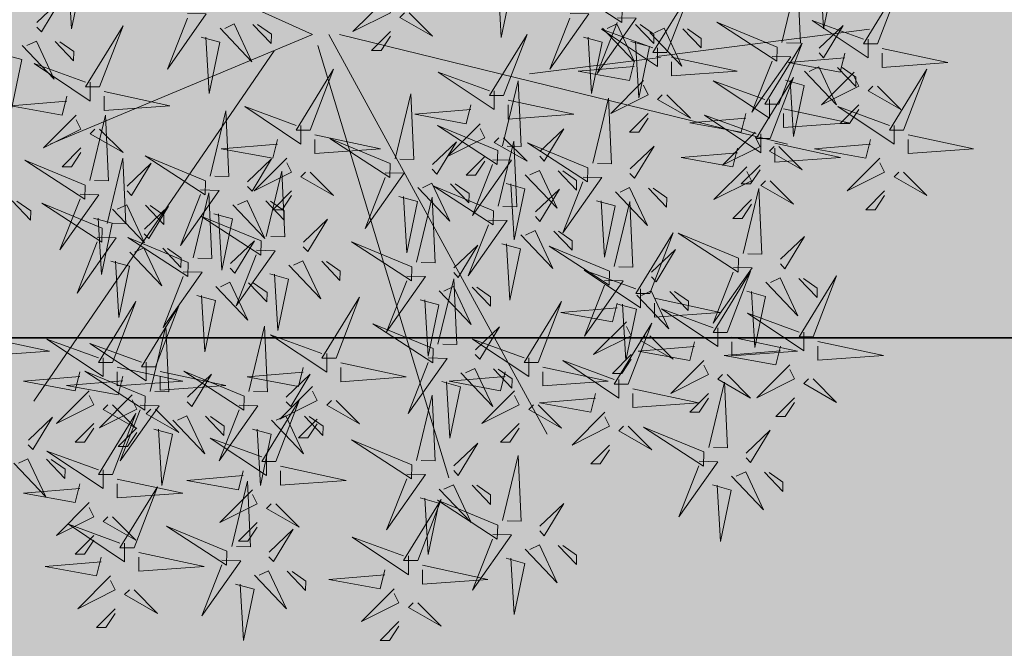
# Model space of a CAD drawing. Units: inches. Extents: x 1704 to 6393, y -157 to 1172.
# Tile 55 of 122: x 1906 to 1931, y 887 to 903. Entities that reach past the tile are written whole.
import ezdxf

# ---------------------------------------------------------------- set-up
doc = ezdxf.new("R2010")
doc.units = ezdxf.units.IN
doc.header["$MEASUREMENT"] = 0
for name, color, linetype, lineweight in [('A-ANNO-DIMS', 7, 'Continuous', 13), ('L-shrub', 74, 'Continuous', 18), ('WALLS', 7, 'Continuous', 35)]:
    doc.layers.add(name, color=color, linetype=linetype, lineweight=lineweight)
doc.layers.add('L-HRDS-PATT', color=9, linetype='Continuous', lineweight=13, true_color=0xc5c1ba)
doc.styles.get("Standard").update_dxf_attribs({"font": 'arial.ttf'})
doc.dimstyles.get("Standard").update_dxf_attribs({"dimtxt": 6, "dimasz": 2, "dimexe": 0.18, "dimexo": 0.0625, "dimgap": 0.09, "dimtad": 0, "dimtih": 1, "dimtoh": 1, "dimdec": 1, "dimzin": 0, "dimdsep": 46, "dimlunit": 3, "dimtxsty": 'Standard', "dimblk": 'ARCHTICK', "dimcen": 0.09, "dimadec": 0, "dimazin": 0, "dimtfac": 1, "dimtdec": 1, "dimtofl": 0, "dimtmove": 0, "dimatfit": 3, "dimfxl": 1, "dimtolj": 1, "dimtzin": 0, "dimarcsym": 0})

# ---------------------------------------------------------------- blocks, each defined once
blk = doc.blocks.new('shrub3')
for p, q in [((-5.99, -2.5), (58.67, 140.12)), ((-14.08, 16.34), (-186.51, 134.74)), ((-5.99, -2.5), (-59.88, 126.66)), ((-11.38, -5.19), (-224.23, -69.78)), ((-5.99, -10.57), (-202.68, -118.21)), ((-5.99, -15.96), (-59.88, -236.62)), ((-17.27, -174.02), (-25.36, -109.43)), ((-16.77, -172.03), (-3.3, -276.98))]:
    blk.add_line(p, q)
for points in [[(-154.93, 159.27), (-161.86, 126.99), (-164.17, 159.27), (-157.24, 159.27)], [(-36.4, 118.43), (-45.64, 120.73), (-41.02, 146.1), (-38.71, 118.43)], [(-15.75, 149.73), (-18.28, 140.55), (-43.52, 145.8), (-15.81, 147.42)], [(-217.01, 144.61), (-233.55, 128.86), (-214.88, 137.63), (-217.07, 142.31)], [(-87.91, 145.34), (-97.36, 136.34), (-92.75, 136.22), (-87.97, 143.03)], [(-227.2, 112.08), (-236.44, 114.38), (-231.82, 139.75), (-229.51, 112.08)], [(-205.66, 137.4), (-194.42, 125.57), (-210.33, 135.21), (-207.96, 137.46)], [(-172.08, 112.08), (-181.32, 114.38), (-176.7, 139.75), (-174.39, 112.08)], [(-80.06, 109.47), (-67.78, 139.19), (-86.97, 109.65), (-80.06, 109.47)], [(-11.37, 140.38), (-27.91, 124.63), (-9.24, 133.4), (-11.43, 138.07)], [(-29.48, 106.9), (-38.71, 106.9), (-20.24, 134.57), (-29.48, 109.2)], [(-0.02, 133.17), (11.22, 121.34), (-4.68, 130.97), (-2.32, 133.22)], [(-263.24, 101.49), (-272.48, 103.79), (-267.86, 129.16), (-265.55, 101.49)], [(-220.28, 100.55), (-229.51, 100.55), (-211.04, 128.22), (-220.28, 102.85)], [(-215.11, 128.4), (-224.56, 119.4), (-219.95, 119.28), (-215.17, 126.09)], [(-165.16, 100.55), (-174.39, 100.55), (-155.92, 128.22), (-165.16, 102.85)], [(-101.26, 101), (-88.98, 130.72), (-108.17, 101.18), (-101.26, 101)], [(-45.64, 113.82), (-61.8, 129.96), (-52.56, 111.51), (-47.94, 113.82)], [(-236.44, 107.46), (-252.6, 123.6), (-243.36, 105.16), (-238.75, 107.46)], [(-181.32, 107.46), (-197.48, 123.6), (-188.24, 105.16), (-183.63, 107.46)], [(-84.61, 111.9), (-84.84, 102.66), (-112.04, 121.82), (-86.91, 111.95)], [(-9.47, 124.17), (-18.92, 115.16), (-14.31, 115.05), (-9.53, 121.86)], [(-256.32, 89.96), (-265.55, 89.96), (-247.08, 117.63), (-256.32, 92.27)], [(-174.2, 90.9), (-183.44, 93.21), (-178.82, 118.57), (-176.51, 90.9)], [(-61.8, 111.51), (-71.03, 120.73), (-71.03, 116.12), (-64.1, 111.51)], [(24.53, 120.08), (22, 110.91), (-3.24, 116.16), (24.47, 117.77)], [(-272.48, 96.88), (-288.64, 113.02), (-279.4, 94.57), (-274.79, 96.88)], [(-252.6, 105.16), (-261.83, 114.38), (-261.83, 109.77), (-254.91, 105.16)], [(-197.48, 105.16), (-206.71, 114.38), (-206.71, 109.77), (-199.79, 105.16)], [(-105.81, 103.43), (-106.04, 94.19), (-133.24, 113.35), (-108.11, 103.48)], [(-183.94, 79.83), (-171.66, 109.54), (-190.85, 80), (-183.94, 79.83)], [(-167.28, 79.37), (-176.51, 79.37), (-158.04, 107.04), (-167.28, 81.68)], [(-77.81, 107.11), (-45.71, 99.37), (-78.04, 97.87), (-77.87, 104.8)], [(-52.56, 102.29), (-64.1, 90.76), (-54.87, 106.9), (-52.56, 104.59)], [(-31.78, 102.29), (-1.77, 90.76), (-31.78, 109.2), (-31.78, 102.29)], [(-288.64, 94.57), (-297.87, 103.79), (-297.87, 99.18), (-290.95, 94.57)], [(-222.59, 95.94), (-192.57, 84.41), (-222.59, 102.85), (-222.59, 95.94)], [(-183.44, 86.29), (-199.6, 102.43), (-190.36, 83.98), (-185.75, 86.29)], [(-167.46, 95.94), (-137.45, 84.41), (-167.46, 102.85), (-167.46, 95.94)], [(-96.31, 105.26), (-98.84, 96.09), (-124.08, 101.34), (-96.37, 102.95)], [(-243.36, 95.94), (-254.91, 84.41), (-245.67, 100.55), (-243.36, 98.24)], [(-188.24, 95.94), (-199.79, 84.41), (-190.55, 100.55), (-188.24, 98.24)], [(-99.01, 98.64), (-66.91, 90.91), (-99.24, 89.41), (-99.07, 96.33)], [(-34.09, 99.98), (-41.02, 67.7), (-43.33, 99.98), (-36.4, 99.98)], [(-258.63, 85.35), (-228.61, 73.82), (-258.63, 92.27), (-258.63, 85.35)], [(-224.89, 93.63), (-231.82, 61.35), (-234.13, 93.63), (-227.2, 93.63)], [(-188.49, 82.25), (-188.72, 73.02), (-215.92, 92.18), (-190.8, 82.31)], [(-199.6, 83.98), (-208.83, 93.21), (-208.83, 88.6), (-201.91, 83.98)], [(-169.77, 93.63), (-176.7, 61.35), (-179.01, 93.63), (-172.08, 93.63)], [(-117.51, 96.79), (-120.04, 87.62), (-145.28, 92.87), (-117.57, 94.48)], [(-91.93, 95.91), (-108.47, 80.16), (-89.8, 88.93), (-91.99, 93.61)], [(-279.4, 85.35), (-290.95, 73.82), (-281.71, 89.96), (-279.4, 87.65)], [(-113.13, 87.44), (-129.67, 71.69), (-111, 80.46), (-113.19, 85.14)], [(-118.22, 58.65), (-105.94, 88.37), (-125.13, 58.83), (-118.22, 58.65)], [(-80.58, 88.7), (-69.34, 76.87), (-85.25, 86.51), (-82.88, 88.76)], [(-260.93, 83.04), (-267.86, 50.76), (-270.17, 83.04), (-263.24, 83.04)], [(-190.36, 74.76), (-201.91, 63.23), (-192.67, 79.37), (-190.36, 77.07)], [(-169.58, 74.76), (-139.57, 63.23), (-169.58, 81.68), (-169.58, 74.76)], [(-101.78, 80.23), (-90.54, 68.4), (-106.45, 78.04), (-104.08, 80.29)], [(-90.03, 79.7), (-99.48, 70.7), (-94.87, 70.58), (-90.09, 77.39)], [(-77.94, 50.18), (-65.66, 79.9), (-84.85, 50.36), (-77.94, 50.18)], [(-200.19, 75.62), (-202.73, 66.44), (-227.97, 71.69), (-200.25, 73.31)], [(-181.69, 77.46), (-149.59, 69.73), (-181.92, 68.23), (-181.75, 75.15)], [(-260.26, 39.6), (-247.98, 69.31), (-267.17, 39.77), (-260.26, 39.6)], [(-171.89, 72.46), (-178.82, 40.17), (-181.13, 72.46), (-174.2, 72.46)], [(-122.77, 61.08), (-123, 51.85), (-150.2, 71), (-125.08, 61.14)], [(-111.23, 71.23), (-120.68, 62.23), (-116.07, 62.11), (-111.29, 68.92)], [(4.43, 58.96), (4.2, 49.73), (-23, 68.88), (2.13, 59.02)], [(-195.81, 66.27), (-212.35, 50.52), (-193.68, 59.29), (-195.87, 63.96)], [(-220.84, 31.61), (-230.08, 33.92), (-225.46, 59.28), (-223.15, 31.61)], [(-183.94, 31.13), (-171.66, 60.84), (-190.85, 31.3), (-183.94, 31.13)], [(-184.46, 59.06), (-173.22, 47.23), (-189.13, 56.86), (-186.76, 59.12)], [(-82.49, 52.61), (-82.72, 43.38), (-109.92, 62.53), (-84.79, 52.67)], [(-134.47, 54.44), (-137, 45.27), (-162.24, 50.52), (-134.53, 52.13)], [(-115.97, 56.29), (-83.87, 48.56), (-116.2, 47.06), (-116.03, 53.98)], [(-264.81, 42.02), (-265.04, 32.79), (-292.24, 51.95), (-267.12, 42.08)], [(-193.91, 50.06), (-203.36, 41.06), (-198.75, 40.94), (-193.97, 47.75)], [(-107.62, 22.66), (-95.34, 52.37), (-114.53, 22.83), (-107.62, 22.66)], [(-7.27, 52.33), (-9.8, 43.15), (-35.04, 48.4), (-7.33, 50.02)], [(-213.92, 20.09), (-223.15, 20.09), (-204.68, 47.76), (-213.92, 22.39)], [(-130.09, 45.1), (-146.63, 29.34), (-127.96, 38.11), (-130.15, 42.79)], [(-94.19, 45.97), (-96.72, 36.8), (-121.96, 42.05), (-94.25, 43.67)], [(-75.69, 47.82), (-43.59, 40.09), (-75.92, 38.59), (-75.75, 45.51)], [(-230.08, 27), (-246.24, 43.14), (-237, 24.7), (-232.39, 27)], [(-188.49, 33.55), (-188.72, 24.32), (-215.92, 43.48), (-190.8, 33.61)], [(-57.6, 14.68), (-66.84, 16.98), (-62.22, 42.34), (-59.91, 14.68)], [(-2.89, 42.98), (-19.43, 27.23), (-0.76, 36), (-2.95, 40.67)], [(-276.51, 35.39), (-279.05, 26.21), (-304.29, 31.46), (-276.57, 33.08)], [(-258.01, 37.23), (-225.91, 29.5), (-258.24, 28), (-258.07, 34.92)], [(-112.17, 25.08), (-112.4, 15.85), (-139.6, 35.01), (-114.47, 25.14)], [(-118.74, 37.88), (-107.5, 26.06), (-123.41, 35.69), (-121.04, 37.94)], [(-89.81, 36.63), (-106.35, 20.87), (-87.68, 29.64), (-89.87, 34.32)], [(-246.24, 24.7), (-255.47, 33.92), (-255.47, 29.31), (-248.55, 24.7)], [(-169.96, 1.97), (-179.2, 4.28), (-174.58, 29.64), (-172.27, 1.97)], [(-78.46, 29.41), (-67.22, 17.59), (-83.13, 27.22), (-80.76, 29.47)], [(-50.68, 3.15), (-59.91, 3.15), (-41.44, 30.82), (-50.68, 5.45)], [(-272.13, 26.04), (-288.67, 10.29), (-270, 19.06), (-272.19, 23.73)], [(-200.19, 26.92), (-202.73, 17.74), (-227.97, 22.99), (-200.25, 24.61)], [(-181.69, 28.76), (-149.59, 21.03), (-181.92, 19.53), (-181.75, 26.45)], [(-128.19, 28.88), (-137.64, 19.88), (-133.03, 19.77), (-128.25, 26.57)], [(-66.84, 10.06), (-83, 26.2), (-73.76, 7.76), (-69.14, 10.06)], [(-0.99, 26.77), (-10.44, 17.76), (-5.83, 17.65), (-1.05, 24.46)], [(-237, 15.47), (-248.55, 3.95), (-239.31, 20.09), (-237, 17.78)], [(-216.23, 15.47), (-186.21, 3.95), (-216.23, 22.39), (-216.23, 15.47)], [(-105.37, 20.29), (-73.27, 12.56), (-105.6, 11.06), (-105.43, 17.99)], [(-87.91, 20.41), (-97.36, 11.41), (-92.75, 11.3), (-87.97, 18.11)], [(-260.78, 18.83), (-249.54, 7), (-265.45, 16.63), (-263.08, 18.88)], [(-195.81, 17.57), (-212.35, 1.82), (-193.68, 10.59), (-195.87, 15.26)], [(-163.04, -9.56), (-172.27, -9.56), (-153.8, 18.11), (-163.04, -7.25)], [(-123.87, 18.45), (-126.4, 9.27), (-151.64, 14.52), (-123.93, 16.14)], [(-83, 7.76), (-92.23, 16.98), (-92.23, 12.37), (-85.3, 7.76)], [(-270.23, 9.83), (-279.68, 0.83), (-275.07, 0.71), (-270.29, 7.52)], [(-218.53, 13.17), (-225.46, -19.11), (-227.77, 13.17), (-220.84, 13.17)], [(-179.2, -2.64), (-195.36, 13.5), (-186.12, -4.95), (-181.51, -2.64)], [(-184.46, 10.36), (-173.22, -1.47), (-189.13, 8.16), (-186.76, 10.41)], [(-119.49, 9.1), (-136.03, -6.65), (-117.36, 2.12), (-119.55, 6.79)], [(-52.98, -1.46), (-22.97, -12.99), (-52.98, 5.45), (-52.98, -1.46)], [(-195.36, -4.95), (-204.59, 4.28), (-204.59, -0.33), (-197.67, -4.95)], [(-193.91, 1.36), (-203.36, -7.64), (-198.75, -7.76), (-193.97, -0.95)], [(-108.14, 1.89), (-96.9, -9.94), (-112.81, -0.3), (-110.44, 1.95)], [(-73.76, -1.46), (-85.3, -12.99), (-76.07, 3.15), (-73.76, 0.84)], [(-55.29, -3.77), (-62.22, -36.05), (-64.53, -3.77), (-57.6, -3.77)], [(-186.12, -14.17), (-197.67, -25.7), (-188.43, -9.56), (-186.12, -11.86)], [(-165.34, -14.17), (-135.33, -25.7), (-165.34, -7.25), (-165.34, -14.17)], [(-117.59, -7.11), (-127.04, -16.11), (-122.43, -16.23), (-117.65, -9.42)], [(-269.6, -38.26), (-278.84, -35.95), (-274.22, -10.59), (-271.91, -38.26)], [(-69.46, -40.86), (-57.18, -11.15), (-76.37, -40.69), (-69.46, -40.86)], [(-167.65, -16.47), (-174.58, -48.76), (-176.89, -16.47), (-169.96, -16.47)], [(-262.68, -49.79), (-271.91, -49.79), (-253.44, -22.12), (-262.68, -47.48)], [(-217.86, -51.45), (-205.58, -21.74), (-224.77, -51.28), (-217.86, -51.45)], [(-120.34, -51.45), (-108.06, -21.74), (-127.25, -51.28), (-120.34, -51.45)], [(11.6, -38.64), (-4.56, -22.5), (4.68, -40.94), (9.3, -38.64)], [(-278.84, -42.87), (-295, -26.73), (-285.76, -45.18), (-281.15, -42.87)], [(-74.01, -38.44), (-74.24, -47.67), (-101.44, -28.52), (-76.31, -38.38)], [(-160.62, -62.04), (-148.34, -32.32), (-167.53, -61.86), (-160.62, -62.04)], [(-4.56, -40.94), (-13.79, -31.72), (-13.79, -36.33), (-6.86, -40.94)], [(-295, -45.18), (-304.23, -35.95), (-304.23, -40.56), (-297.31, -45.18)], [(-222.41, -49.03), (-222.64, -58.26), (-249.84, -39.1), (-224.72, -48.97)], [(-124.89, -49.03), (-125.12, -58.26), (-152.32, -39.1), (-127.2, -48.97)], [(-67.21, -43.23), (-35.11, -50.96), (-67.44, -52.46), (-67.27, -45.54)], [(-264.99, -54.4), (-234.97, -65.93), (-264.99, -47.48), (-264.99, -54.4)], [(-85.71, -45.07), (-88.24, -54.25), (-113.48, -49), (-85.77, -47.38)], [(4.68, -50.16), (-6.86, -61.69), (2.37, -45.55), (4.68, -47.86)], [(-285.76, -54.4), (-297.31, -65.93), (-288.07, -49.79), (-285.76, -52.09)], [(-165.17, -59.61), (-165.4, -68.85), (-192.6, -49.69), (-167.48, -59.56)], [(-40.64, -80.61), (-49.88, -78.3), (-45.26, -52.94), (-42.95, -80.61)], [(-267.29, -56.71), (-274.22, -88.99), (-276.53, -56.71), (-269.6, -56.71)], [(-234.11, -55.66), (-236.65, -64.84), (-261.89, -59.59), (-234.17, -57.97)], [(-215.61, -53.82), (-183.51, -61.55), (-215.84, -63.05), (-215.67, -56.12)], [(-136.59, -55.66), (-139.12, -64.84), (-164.36, -59.59), (-136.65, -57.97)], [(-118.09, -53.82), (-85.99, -61.55), (-118.32, -63.05), (-118.15, -56.12)], [(-81.33, -54.42), (-97.87, -70.17), (-79.2, -61.4), (-81.39, -56.73)], [(-92.78, -91.68), (-80.5, -61.97), (-99.69, -91.51), (-92.78, -91.68)], [(-69.98, -61.63), (-58.74, -73.46), (-74.65, -63.83), (-72.28, -61.58)], [(-247.54, -93.8), (-235.26, -64.08), (-254.45, -93.62), (-247.54, -93.8)], [(-229.73, -65.01), (-246.27, -80.76), (-227.6, -71.99), (-229.79, -67.32)], [(-176.87, -66.25), (-179.4, -75.42), (-204.64, -70.17), (-176.93, -68.56)], [(-158.37, -64.4), (-126.27, -72.13), (-158.6, -73.63), (-158.43, -66.71)], [(-132.21, -65.01), (-148.75, -80.76), (-130.08, -71.99), (-132.27, -67.32)], [(-63.1, -93.8), (-50.82, -64.08), (-70.01, -93.62), (-63.1, -93.8)], [(-33.72, -92.14), (-42.95, -92.14), (-24.48, -64.47), (-33.72, -89.83)], [(-218.38, -72.22), (-207.14, -84.05), (-223.05, -74.41), (-220.68, -72.16)], [(-172.08, -97.55), (-181.32, -95.24), (-176.7, -69.88), (-174.39, -97.55)], [(-120.86, -72.22), (-109.62, -84.05), (-125.53, -74.41), (-123.16, -72.16)], [(-79.43, -70.63), (-88.88, -79.64), (-84.27, -79.75), (-79.49, -72.94)], [(-49.88, -85.22), (-66.04, -69.08), (-56.8, -87.52), (-52.18, -85.22)], [(-172.49, -75.6), (-189.03, -91.35), (-170.36, -82.58), (-172.55, -77.9)], [(-252.09, -91.37), (-252.32, -100.61), (-279.52, -81.45), (-254.4, -91.32)], [(-227.83, -81.22), (-237.28, -90.22), (-232.67, -90.34), (-227.89, -83.53)], [(-165.16, -109.08), (-174.39, -109.08), (-155.92, -81.41), (-165.16, -106.77)], [(-130.31, -81.22), (-139.76, -90.22), (-135.15, -90.34), (-130.37, -83.53)], [(-97.33, -89.26), (-97.56, -98.49), (-124.76, -79.33), (-99.63, -89.2)], [(-67.65, -91.37), (-67.88, -100.61), (-95.08, -81.45), (-69.95, -91.32)], [(-66.04, -87.52), (-75.27, -78.3), (-75.27, -82.91), (-68.34, -87.52)], [(-181.32, -102.16), (-197.48, -86.02), (-188.24, -104.46), (-183.63, -102.16)], [(-161.14, -82.81), (-149.9, -94.64), (-165.81, -85), (-163.44, -82.75)], [(-170.59, -91.81), (-180.04, -100.81), (-175.43, -100.93), (-170.65, -94.12)], [(-56.8, -96.75), (-68.34, -108.28), (-59.11, -92.14), (-56.8, -94.44)], [(-36.02, -96.75), (-6.01, -108.28), (-36.02, -89.83), (-36.02, -96.75)], [(20.29, -91.66), (17.76, -100.83), (-7.48, -95.58), (20.23, -93.97)], [(-245.29, -96.16), (-213.19, -103.89), (-245.52, -105.4), (-245.35, -98.47)], [(-197.48, -104.46), (-206.71, -95.24), (-206.71, -99.85), (-199.79, -104.46)], [(-109.03, -95.89), (-111.56, -105.07), (-136.8, -99.82), (-109.09, -98.2)], [(-90.53, -94.05), (-58.43, -101.78), (-90.76, -103.28), (-90.59, -96.35)], [(-60.85, -96.16), (-28.75, -103.89), (-61.08, -105.4), (-60.91, -98.47)], [(-263.79, -98.01), (-266.33, -107.18), (-291.57, -101.93), (-263.85, -100.32)], [(-79.35, -98.01), (-81.88, -107.18), (-107.12, -101.93), (-79.41, -100.32)], [(-38.33, -99.05), (-45.26, -131.33), (-47.57, -99.05), (-40.64, -99.05)], [(-104.65, -105.24), (-121.19, -120.99), (-102.52, -112.22), (-104.71, -107.55)], [(-259.41, -107.36), (-275.95, -123.11), (-257.28, -114.34), (-259.47, -109.66)], [(-188.24, -113.69), (-199.79, -125.22), (-190.55, -109.08), (-188.24, -111.38)], [(-167.46, -113.69), (-137.45, -125.22), (-167.46, -106.77), (-167.46, -113.69)], [(-74.97, -107.36), (-91.51, -123.11), (-72.84, -114.34), (-75.03, -109.66)], [(-71.58, -138.26), (-59.3, -108.55), (-78.49, -138.09), (-71.58, -138.26)], [(-248.06, -114.57), (-236.82, -126.4), (-252.73, -116.76), (-250.36, -114.51)], [(-182.68, -142.01), (-191.92, -139.71), (-187.3, -114.34), (-184.99, -142.01)], [(-169.77, -115.99), (-176.7, -148.27), (-179.01, -115.99), (-172.08, -115.99)], [(-93.3, -112.45), (-82.06, -124.28), (-97.97, -114.64), (-95.6, -112.39)], [(-63.62, -114.57), (-52.38, -126.4), (-68.29, -116.76), (-65.92, -114.51)], [(-122.46, -148.85), (-110.18, -119.14), (-129.37, -148.68), (-122.46, -148.85)], [(4.43, -129.49), (4.2, -138.72), (-23, -119.56), (2.13, -129.43)], [(-257.51, -123.57), (-266.96, -132.57), (-262.35, -132.69), (-257.57, -125.88)], [(-175.76, -153.54), (-184.99, -153.54), (-166.52, -125.87), (-175.76, -151.23)], [(-138.16, -152.6), (-147.4, -150.29), (-142.78, -124.93), (-140.47, -152.6)], [(-102.75, -121.45), (-112.2, -130.45), (-107.59, -130.57), (-102.81, -123.76)], [(-76.13, -135.84), (-76.36, -145.07), (-103.56, -125.92), (-78.43, -135.78)], [(-73.07, -123.57), (-82.52, -132.57), (-77.91, -132.69), (-73.13, -125.88)], [(6.86, -155.2), (19.14, -125.49), (-0.05, -155.03), (6.86, -155.2)], [(-191.92, -146.62), (-208.08, -130.48), (-198.84, -148.93), (-194.23, -146.62)], [(-19.44, -161.07), (-28.68, -158.76), (-24.06, -133.4), (-21.75, -161.07)], [(-208.08, -148.93), (-217.31, -139.71), (-217.31, -144.32), (-210.39, -148.93)], [(-127.01, -146.43), (-127.24, -155.66), (-154.44, -136.5), (-129.32, -146.37)], [(-131.24, -164.13), (-140.47, -164.13), (-122, -136.46), (-131.24, -161.82)], [(-69.33, -140.63), (-37.23, -148.36), (-69.56, -149.86), (-69.39, -142.94)], [(-7.27, -136.12), (-9.8, -145.3), (-35.04, -140.05), (-7.33, -138.43)], [(-147.4, -157.21), (-163.56, -141.07), (-154.32, -159.52), (-149.71, -157.21)], [(-87.83, -142.48), (-90.36, -151.65), (-115.6, -146.4), (-87.89, -144.78)], [(2.31, -152.78), (2.08, -162.01), (-25.12, -142.86), (0.01, -152.72)], [(-12.52, -172.6), (-21.75, -172.6), (-3.28, -144.93), (-12.52, -170.29)], [(-2.89, -145.47), (-19.43, -161.22), (-0.76, -152.45), (-2.95, -147.78)], [(-163.56, -159.52), (-172.79, -150.29), (-172.79, -154.9), (-165.87, -159.52)], [(-28.68, -165.68), (-44.84, -149.54), (-35.6, -167.99), (-30.98, -165.68)], [(-198.84, -158.15), (-210.39, -169.68), (-201.15, -153.54), (-198.84, -155.85)], [(-178.06, -158.15), (-148.05, -169.68), (-178.06, -151.23), (-178.06, -158.15)], [(-138.71, -153.06), (-141.24, -162.24), (-166.48, -156.99), (-138.77, -155.37)], [(-120.21, -151.22), (-88.11, -158.95), (-120.44, -160.45), (-120.27, -153.52)], [(-83.45, -151.82), (-99.99, -167.57), (-81.32, -158.8), (-83.51, -154.13)], [(-72.1, -159.03), (-60.86, -170.86), (-76.77, -161.23), (-74.4, -158.98)], [(-44.84, -167.99), (-54.07, -158.76), (-54.07, -163.37), (-47.14, -167.99)], [(-9.39, -159.41), (-11.92, -168.59), (-37.16, -163.34), (-9.45, -161.72)], [(-180.37, -160.46), (-187.3, -192.74), (-189.61, -160.46), (-182.68, -160.46)], [(-157.24, -190.71), (-166.48, -188.41), (-161.86, -163.04), (-159.55, -190.71)], [(-154.32, -168.74), (-165.87, -180.27), (-156.63, -164.13), (-154.32, -166.43)], [(-134.33, -162.41), (-150.87, -178.16), (-132.2, -169.39), (-134.39, -164.72)], [(-133.54, -168.74), (-103.53, -180.27), (-133.54, -161.82), (-133.54, -168.74)], [(-0.99, -161.68), (-10.44, -170.68), (-5.83, -170.8), (-1.05, -163.99)], [(-211.5, -195.43), (-199.22, -165.72), (-218.41, -195.26), (-211.5, -195.43)], [(-122.98, -169.62), (-111.74, -181.45), (-127.65, -171.81), (-125.28, -169.56)], [(-81.55, -168.04), (-91, -177.04), (-86.39, -177.15), (-81.61, -170.34)], [(-5.01, -168.76), (-21.55, -184.51), (-2.88, -175.74), (-5.07, -171.07)], [(-150.32, -202.24), (-159.55, -202.24), (-141.08, -174.57), (-150.32, -199.93)], [(-135.85, -171.04), (-142.78, -203.33), (-145.09, -171.04), (-138.16, -171.04)], [(-35.6, -177.21), (-47.14, -188.74), (-37.91, -172.6), (-35.6, -174.9)], [(-14.82, -177.21), (15.19, -188.74), (-14.82, -170.29), (-14.82, -177.21)], [(-166.48, -195.32), (-182.64, -179.18), (-173.4, -197.63), (-168.79, -195.32)], [(-132.43, -178.62), (-141.88, -187.62), (-137.27, -187.74), (-132.49, -180.93)], [(-216.05, -193.01), (-216.28, -202.24), (-243.48, -183.09), (-218.36, -192.95)], [(-116.1, -212.37), (-103.82, -182.66), (-123.01, -212.2), (-116.1, -212.37)], [(-61.84, -211.89), (-71.08, -209.58), (-66.46, -184.22), (-64.15, -211.89)], [(-17.13, -179.51), (-24.06, -211.79), (-26.37, -179.51), (-19.44, -179.51)], [(-182.64, -197.63), (-191.87, -188.41), (-191.87, -193.02), (-184.95, -197.63)], [(-44.88, -216.12), (-54.12, -213.81), (-49.5, -188.45), (-47.19, -216.12)], [(-3.11, -184.97), (-12.56, -193.97), (-7.95, -194.09), (-3.17, -187.28)], [(-209.25, -197.8), (-177.15, -205.53), (-209.48, -207.03), (-209.31, -200.11)], [(-54.92, -223.41), (-64.15, -223.41), (-45.68, -195.75), (-54.92, -221.11)], [(-227.75, -199.64), (-230.29, -208.82), (-255.53, -203.57), (-227.81, -201.95)], [(-173.4, -206.85), (-184.95, -218.38), (-175.71, -202.24), (-173.4, -204.55)], [(-152.62, -206.85), (-122.61, -218.38), (-152.62, -199.93), (-152.62, -206.85)], [(-120.65, -209.95), (-120.88, -219.18), (-148.08, -200.02), (-122.96, -209.89)], [(-71.08, -216.5), (-87.24, -200.36), (-78, -218.8), (-73.38, -216.5)], [(-37.96, -227.65), (-47.19, -227.65), (-28.72, -199.98), (-37.96, -225.34)], [(-12.22, -231.43), (0.06, -201.71), (-19.13, -231.26), (-12.22, -231.43)], [(-159.36, -233.06), (-168.6, -230.75), (-163.98, -205.39), (-161.67, -233.06)], [(-54.12, -220.73), (-70.28, -204.59), (-61.04, -223.04), (-56.42, -220.73)], [(-223.37, -208.99), (-239.91, -224.74), (-221.24, -215.97), (-223.43, -211.3)], [(-154.93, -209.16), (-161.86, -241.44), (-164.17, -209.16), (-157.24, -209.16)], [(-87.24, -218.8), (-96.47, -209.58), (-96.47, -214.19), (-89.54, -218.8)], [(-212.02, -216.2), (-200.78, -228.03), (-216.69, -218.4), (-214.32, -216.15)], [(-152.44, -244.59), (-161.67, -244.59), (-143.2, -216.92), (-152.44, -242.28)], [(-132.35, -216.58), (-134.88, -225.76), (-160.12, -220.51), (-132.41, -218.89)], [(-113.85, -214.74), (-81.75, -222.47), (-114.08, -223.97), (-113.91, -217.05)], [(-70.28, -223.04), (-79.51, -213.81), (-79.51, -218.43), (-72.58, -223.04)], [(-168.6, -237.67), (-184.76, -221.53), (-175.52, -239.98), (-170.91, -237.67)], [(-57.22, -228.03), (-27.21, -239.55), (-57.22, -221.11), (-57.22, -228.03)], [(-16.77, -229.01), (-17, -238.24), (-44.2, -219.08), (-19.07, -228.95)], [(-221.47, -225.2), (-230.92, -234.21), (-226.31, -234.32), (-221.53, -227.51)], [(-127.97, -225.93), (-144.51, -241.68), (-125.84, -232.91), (-128.03, -228.24)], [(-78, -228.03), (-89.54, -239.55), (-80.31, -223.41), (-78, -225.72)], [(-61.04, -232.26), (-72.58, -243.79), (-63.35, -227.65), (-61.04, -229.95)], [(-40.26, -232.26), (-10.25, -243.79), (-40.26, -225.34), (-40.26, -232.26)], [(-184.76, -239.98), (-193.99, -230.75), (-193.99, -235.37), (-187.07, -239.98)], [(-59.53, -230.33), (-66.46, -262.61), (-68.77, -230.33), (-61.84, -230.33)], [(-116.62, -233.14), (-105.38, -244.97), (-121.29, -235.34), (-118.92, -233.09)], [(-28.47, -235.64), (-31, -244.81), (-56.24, -239.56), (-28.53, -237.95)], [(-42.57, -234.57), (-49.5, -266.85), (-51.81, -234.57), (-44.88, -234.57)], [(-15.2, -264.82), (-24.44, -262.51), (-19.82, -237.15), (-17.51, -264.82)], [(-9.97, -233.79), (22.13, -241.53), (-10.2, -243.03), (-10.03, -236.1)], [(-154.74, -249.2), (-124.73, -260.73), (-154.74, -242.28), (-154.74, -249.2)], [(-126.07, -242.14), (-135.52, -251.14), (-130.91, -251.26), (-126.13, -244.45)], [(-175.52, -249.2), (-187.07, -260.73), (-177.83, -244.59), (-175.52, -246.89)], [(-24.09, -244.99), (-40.63, -260.74), (-21.96, -251.97), (-24.15, -247.3)], [(-157.05, -251.51), (-163.98, -283.79), (-166.29, -251.51), (-159.36, -251.51)], [(-57.6, -277.52), (-66.84, -275.22), (-62.22, -249.86), (-59.91, -277.52)], [(-8.28, -276.35), (-17.51, -276.35), (0.96, -248.68), (-8.28, -274.04)], [(-12.74, -252.2), (-1.5, -264.03), (-17.4, -254.39), (-15.04, -252.14)], [(24.53, -250.46), (22, -259.64), (-3.24, -254.39), (24.47, -252.77)], [(-24.44, -269.43), (-40.6, -253.29), (-31.36, -271.74), (-26.74, -269.43)], [(-50.68, -289.05), (-59.91, -289.05), (-41.44, -261.38), (-50.68, -286.75)], [(-22.19, -261.2), (-31.64, -270.2), (-27.03, -270.32), (-22.25, -263.51)], [(-66.84, -282.14), (-83, -266), (-73.76, -284.44), (-69.14, -282.14)], [(-40.6, -271.74), (-49.83, -262.51), (-49.83, -267.13), (-42.9, -271.74)], [(-83, -284.44), (-92.23, -275.22), (-92.23, -279.83), (-85.3, -284.44)], [(-31.36, -280.96), (-42.9, -292.49), (-33.67, -276.35), (-31.36, -278.65)], [(-10.58, -280.96), (19.43, -292.49), (-10.58, -274.04), (-10.58, -280.96)], [(-12.89, -283.27), (-19.82, -315.55), (-22.13, -283.27), (-15.2, -283.27)], [(-73.76, -293.67), (-85.3, -305.19), (-76.07, -289.05), (-73.76, -291.36)], [(-52.98, -293.67), (-22.97, -305.19), (-52.98, -286.75), (-52.98, -293.67)], [(-55.29, -295.97), (-62.22, -328.25), (-64.53, -295.97), (-57.6, -295.97)]]:
    blk.add_lwpolyline(points)
blk = doc.blocks.new('_ArchTick')
at = {"color": 0, "linetype": 'ByBlock', "const_width": 0.15}
blk.add_lwpolyline([(-0.5, -0.5), (0.5, 0.5)], dxfattribs=at)
blk = doc.blocks.new('*D93')
at = {"layer": 'A-ANNO-DIMS', "color": 0, "lineweight": -2, "transparency": 16777216}
for p, q in [((2605.286, 895.213), (1829.698, 895.213)), ((1829.878, 895.213), (1829.878, 495.866)), ((1829.878, 90.213), (1829.878, 489.56)), ((2605.286, 90.213), (1829.698, 90.213))]:
    blk.add_line(p, q, dxfattribs=at)
at = {"layer": 'Defpoints', "color": 0, "lineweight": -3, "transparency": 16777216}
for p in [(2605.349, 895.213), (1829.878, 90.213), (2605.349, 90.213)]:
    blk.add_point(p, dxfattribs=at)
at = {"layer": 'A-ANNO-DIMS', "color": 0, "lineweight": -2, "transparency": 16777216, "xscale": 2, "yscale": 2, "zscale": 2}
for p, rotation in [((1829.878, 895.213), 90), ((1829.878, 90.213), 270)]:
    blk.add_blockref('_ArchTick', p, dxfattribs=dict(at, rotation=rotation))
at = {"layer": 'A-ANNO-DIMS', "color": 0, "transparency": 16777216, "insert": (1829.878, 492.713), "char_height": 6, "attachment_point": 5}
blk.add_mtext('\\A1;805', dxfattribs=at)
blk = doc.blocks.new('*D94')
at = {"layer": 'A-ANNO-DIMS', "color": 0, "lineweight": -2, "transparency": 16777216}
for p, q in [((1898.349, 895.275), (1898.349, 1105.287)), ((1898.349, 1105.107), (1979.39, 1105.107)), ((2073.349, 1105.107), (1992.307, 1105.107)), ((2073.349, 895.275), (2073.349, 1105.287))]:
    blk.add_line(p, q, dxfattribs=at)
at = {"layer": 'Defpoints', "color": 0, "lineweight": -3, "transparency": 16777216}
for p in [(2073.349, 1105.107), (1898.349, 895.213), (2073.349, 895.213)]:
    blk.add_point(p, dxfattribs=at)
at = {"layer": 'A-ANNO-DIMS', "color": 0, "lineweight": -2, "transparency": 16777216, "xscale": 2, "yscale": 2, "zscale": 2, "rotation": 180}
blk.add_blockref('_ArchTick', (1898.349, 1105.107), dxfattribs=at)
at = {"layer": 'A-ANNO-DIMS', "color": 0, "lineweight": -2, "transparency": 16777216, "xscale": 2, "yscale": 2, "zscale": 2}
blk.add_blockref('_ArchTick', (2073.349, 1105.107), dxfattribs=at)
at = {"layer": 'A-ANNO-DIMS', "color": 0, "transparency": 16777216, "insert": (1985.849, 1105.107), "char_height": 6, "attachment_point": 5}
blk.add_mtext('\\A1;175', dxfattribs=at)

msp = doc.modelspace()

# ---------------------------------------------------------------- hatches: boundary and pattern name
at = {"layer": 'L-HRDS-PATT', "transparency": 33554643}
h = msp.add_hatch(color=256, dxfattribs=at)
h.dxf.hatch_style = 1
h.paths.add_polyline_path([(2065.589, 1033.213), (1898.349, 1033.213), (1898.349, 895.213), (2065.589, 895.213)])
h = msp.add_hatch(color=256, dxfattribs=at)
h.dxf.hatch_style = 1
h.paths.add_polyline_path([(2073.349, 719.213), (2021.151, 719.213), (2021.151, 711.213), (2073.349, 711.213)])
h.paths.add_polyline_path([(1977.349, 719.213), (1969.349, 719.213), (1898.349, 719.213), (1898.349, 711.213), (1977.349, 711.213)])
h.paths.add_polyline_path([(1977.349, 895.213), (1898.349, 895.213), (1898.349, 887.213), (1969.349, 887.213), (1977.349, 887.213)])

# ---------------------------------------------------------------- linework, layer by layer
at = {"layer": 'WALLS'}
msp.add_line((2167.349, 895.213), (1898.349, 895.213), dxfattribs=at)

# ---------------------------------------------------------------- block references
at = {"layer": 'L-shrub', "xscale": 0.0510581485411622, "yscale": 0.0510581485411622, "zscale": 0.0510581485411622, "rotation": 89.99999999999996}
msp.add_blockref('shrub3', (1913.464, 903.144), dxfattribs=at)

# ---------------------------------------------------------------- dimensions: what is measured, and where the dimension line sits
at = {"layer": 'A-ANNO-DIMS'}
dim = msp.add_linear_dim(base=(2073.349, 1105.107), p1=(1898.349, 895.213), p2=(2073.349, 895.213), dimstyle='Standard', override={"dimdec": 0, "dimlfac": 1, "dimrnd": 0, "dimzin": 0, "dimdsep": 46, "dimlunit": 2}, dxfattribs=at)
dim.commit()
dim.dimension.update_dxf_attribs({"geometry": '*D94', "text_midpoint": (1985.849, 1105.107)})
dim = msp.add_linear_dim(base=(1829.878, 90.213), p1=(2605.349, 895.213), p2=(2605.349, 90.213), angle=90, dimstyle='Standard', override={"dimdec": 0, "dimlfac": 1, "dimrnd": 0, "dimzin": 0, "dimdsep": 46, "dimlunit": 2}, dxfattribs=at)
dim.commit()
dim.dimension.update_dxf_attribs({"geometry": '*D93', "text_midpoint": (1829.878, 492.713)})

doc.saveas('drawing.dxf')
